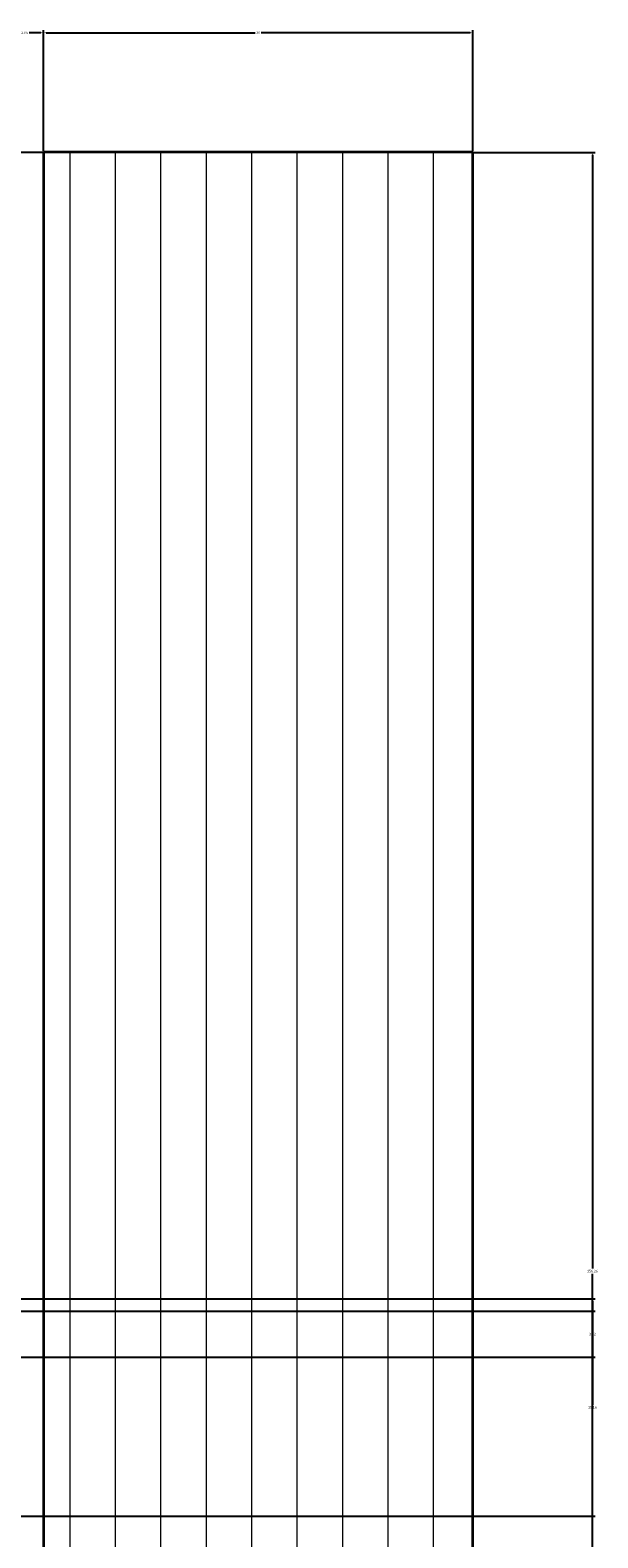
# Model space of a CAD drawing. Units: millimetres. Extents: x 446512 to 447461, y 70395 to 70610.
# Tile 21 of 39: x 446748 to 446788, y 70473 to 70578. Entities that reach past the tile are written whole.
import ezdxf

# ---------------------------------------------------------------- set-up
doc = ezdxf.new("R2010")
doc.units = ezdxf.units.MM
for name, color, linetype, lineweight in [('A-ANNO-DIMS', 2, 'Continuous', 18), ('A-FURN', 7, 'Continuous', 35), ('A-FURN-PATT', 38, 'Continuous', 13)]:
    doc.layers.add(name, color=color, linetype=linetype, lineweight=lineweight)
doc.styles.get("Standard").update_dxf_attribs({"font": 'arial.ttf'})
doc.dimstyles.get("Standard").update_dxf_attribs({"dimtxt": 0.18, "dimasz": 0.18, "dimexe": 0.18, "dimexo": 0.0625, "dimgap": 0.09, "dimtad": 0, "dimtih": 1, "dimtoh": 1, "dimdec": 4, "dimzin": 0, "dimdsep": 46, "dimtxsty": 'Standard', "dimcen": 0.09, "dimadec": 0, "dimazin": 0, "dimtfac": 1, "dimtdec": 4, "dimtofl": 0, "dimtmove": 0, "dimatfit": 3, "dimfxl": 1, "dimtolj": 1, "dimtzin": 0, "dimarcsym": 0})

# ---------------------------------------------------------------- blocks, each defined once
blk = doc.blocks.new('*D15')
at = {"layer": 'A-ANNO-DIMS', "color": 0, "lineweight": -2, "transparency": 16777216}
for p, q in [((446746.57, 70533.44), (446746.57, 70578.17)), ((446749.22, 70569.71), (446749.22, 70578.17)), ((446746.75, 70577.99), (446747.57, 70577.99)), ((446749.04, 70577.99), (446748.22, 70577.99))]:
    blk.add_line(p, q, dxfattribs=at)
at = {"layer": 'A-ANNO-DIMS', "color": 0, "transparency": 16777216}
for points in [[(446746.75, 70578.02), (446746.75, 70577.96), (446746.57, 70577.99)], [(446749.04, 70578.02), (446749.04, 70577.96), (446749.22, 70577.99)]]:
    blk.add_solid(points, dxfattribs=at)
at = {"layer": 'Defpoints', "color": 0, "transparency": 16777216}
for p in [(446749.22, 70577.99), (446749.22, 70569.64), (446746.57, 70533.38)]:
    blk.add_point(p, dxfattribs=at)
at = {"layer": 'A-ANNO-DIMS', "color": 0, "transparency": 16777216, "insert": (446747.9, 70577.99), "char_height": 0.18, "attachment_point": 5}
blk.add_mtext('\\A1;2.65', dxfattribs=at)
blk = doc.blocks.new('*D16')
at = {"layer": 'A-ANNO-DIMS', "color": 0, "lineweight": -2, "transparency": 16777216}
for p, q in [((446749.22, 70569.71), (446749.22, 70578.17)), ((446779.22, 70569.71), (446779.22, 70578.17)), ((446749.4, 70577.99), (446764, 70577.99)), ((446779.04, 70577.99), (446764.44, 70577.99))]:
    blk.add_line(p, q, dxfattribs=at)
at = {"layer": 'A-ANNO-DIMS', "color": 0, "transparency": 16777216}
for points in [[(446749.4, 70578.02), (446749.4, 70577.96), (446749.22, 70577.99)], [(446779.04, 70578.02), (446779.04, 70577.96), (446779.22, 70577.99)]]:
    blk.add_solid(points, dxfattribs=at)
at = {"layer": 'Defpoints', "color": 0, "transparency": 16777216}
for p in [(446779.22, 70577.99), (446749.22, 70569.64), (446779.22, 70569.64)]:
    blk.add_point(p, dxfattribs=at)
at = {"layer": 'A-ANNO-DIMS', "color": 0, "transparency": 16777216, "insert": (446764.22, 70577.99), "char_height": 0.18, "attachment_point": 5}
blk.add_mtext('\\A1;30', dxfattribs=at)
blk = doc.blocks.new('*D17')
at = {"layer": 'A-ANNO-DIMS', "color": 0, "lineweight": -2, "transparency": 16777216}
for p, q in [((446779.29, 70569.64), (446787.75, 70569.64)), ((446787.57, 70569.46), (446787.57, 70491.7)), ((446787.57, 70413.56), (446787.57, 70491.33)), ((446779.29, 70413.38), (446787.75, 70413.38))]:
    blk.add_line(p, q, dxfattribs=at)
at = {"layer": 'A-ANNO-DIMS', "color": 0, "transparency": 16777216}
for points in [[(446787.54, 70569.46), (446787.6, 70569.46), (446787.57, 70569.64)], [(446787.54, 70413.56), (446787.6, 70413.56), (446787.57, 70413.38)]]:
    blk.add_solid(points, dxfattribs=at)
at = {"layer": 'Defpoints', "color": 0, "transparency": 16777216}
for p in [(446779.22, 70569.64), (446787.57, 70569.64), (446779.22, 70413.38)]:
    blk.add_point(p, dxfattribs=at)
at = {"layer": 'A-ANNO-DIMS', "color": 0, "transparency": 16777216, "insert": (446787.57, 70491.51), "char_height": 0.18, "attachment_point": 5}
blk.add_mtext('\\A1;156.26', dxfattribs=at)
blk = doc.blocks.new('*D24')
at = {"layer": 'A-ANNO-DIMS', "color": 0, "lineweight": -2, "transparency": 16777216}
for p, q in [((446749.16, 70569.64), (446678.04, 70569.64)), ((446678.22, 70569.46), (446678.22, 70551.7)), ((446678.22, 70533.56), (446678.22, 70551.33)), ((446686.51, 70533.38), (446678.04, 70533.38))]:
    blk.add_line(p, q, dxfattribs=at)
at = {"layer": 'A-ANNO-DIMS', "color": 0, "transparency": 16777216}
for points in [[(446678.19, 70569.46), (446678.25, 70569.46), (446678.22, 70569.64)], [(446678.19, 70533.56), (446678.25, 70533.56), (446678.22, 70533.38)]]:
    blk.add_solid(points, dxfattribs=at)
at = {"layer": 'Defpoints', "color": 0, "transparency": 16777216}
for p in [(446678.22, 70569.64), (446749.22, 70569.64), (446686.57, 70533.38)]:
    blk.add_point(p, dxfattribs=at)
at = {"layer": 'A-ANNO-DIMS', "color": 0, "transparency": 16777216, "insert": (446678.22, 70551.51), "char_height": 0.18, "attachment_point": 5}
blk.add_mtext('\\A1;36.26', dxfattribs=at)
blk = doc.blocks.new('*D30')
at = {"layer": 'A-ANNO-DIMS', "color": 0, "lineweight": -2, "transparency": 16777216}
for p, q in [((446743.64, 70489.58), (446787.75, 70489.58)), ((446787.57, 70489.4), (446787.57, 70482.18)), ((446787.57, 70474.58), (446787.57, 70481.81)), ((446743.64, 70474.4), (446787.75, 70474.4))]:
    blk.add_line(p, q, dxfattribs=at)
at = {"layer": 'A-ANNO-DIMS', "color": 0, "transparency": 16777216}
for points in [[(446787.54, 70489.4), (446787.6, 70489.4), (446787.57, 70489.58)], [(446787.54, 70474.58), (446787.6, 70474.58), (446787.57, 70474.4)]]:
    blk.add_solid(points, dxfattribs=at)
at = {"layer": 'Defpoints', "color": 0, "transparency": 16777216}
for p in [(446743.58, 70489.58), (446787.57, 70489.58), (446743.58, 70474.4)]:
    blk.add_point(p, dxfattribs=at)
at = {"layer": 'A-ANNO-DIMS', "color": 0, "transparency": 16777216, "insert": (446787.57, 70481.99), "char_height": 0.18, "attachment_point": 5}
blk.add_mtext('\\A1;15.18', dxfattribs=at)
blk = doc.blocks.new('*D35')
at = {"layer": 'A-ANNO-DIMS', "color": 0, "lineweight": -2, "transparency": 16777216}
for p, q in [((446742.78, 70488.72), (446787.75, 70488.72)), ((446787.57, 70488.54), (446787.57, 70487.3)), ((446787.57, 70485.68), (446787.57, 70486.93)), ((446739.38, 70485.5), (446787.75, 70485.5))]:
    blk.add_line(p, q, dxfattribs=at)
at = {"layer": 'A-ANNO-DIMS', "color": 0, "transparency": 16777216}
for points in [[(446787.54, 70488.54), (446787.6, 70488.54), (446787.57, 70488.72)], [(446787.54, 70485.68), (446787.6, 70485.68), (446787.57, 70485.5)]]:
    blk.add_solid(points, dxfattribs=at)
at = {"layer": 'Defpoints', "color": 0, "transparency": 16777216}
for p in [(446742.72, 70488.72), (446739.32, 70485.5), (446787.57, 70485.5)]:
    blk.add_point(p, dxfattribs=at)
at = {"layer": 'A-ANNO-DIMS', "color": 0, "transparency": 16777216, "insert": (446787.57, 70487.11), "char_height": 0.18, "attachment_point": 5}
blk.add_mtext('\\A1;3.22', dxfattribs=at)

msp = doc.modelspace()

# ---------------------------------------------------------------- hatches: boundary and pattern name
at = {"layer": 'A-FURN-PATT'}
h = msp.add_hatch(dxfattribs=at)
h.set_pattern_fill('ANSI31', color=256, angle=45)
h.paths.add_polyline_path([(446779.2235, 70569.6449), (446749.2235, 70569.6449), (446749.2235, 70413.3815), (446779.2235, 70413.3815)])

# ---------------------------------------------------------------- linework, layer by layer
at = {"layer": 'A-FURN'}
for p, q in [((446779.2235, 70569.6449), (446749.2235, 70569.6449)), ((446749.2235, 70569.6449), (446749.2235, 70413.3815)), ((446779.2235, 70413.3815), (446779.2235, 70569.6449))]:
    msp.add_line(p, q, dxfattribs=at)

# ---------------------------------------------------------------- dimensions: what is measured, and where the dimension line sits
at = {"layer": 'A-ANNO-DIMS'}
for base, p1, p2, override, picture, middle in [((446749.2235, 70577.9949), (446746.5728, 70533.3816), (446749.2235, 70569.6449), {"dimdec": 2, "dimlfac": 1, "dimrnd": 0, "dimzin": 0, "dimdsep": 46, "dimlunit": 2}, '*D15', (446747.8982, 70577.9949)), ((446779.2235, 70577.9949), (446749.2235, 70569.6449), (446779.2235, 70569.6449), {"dimdec": 0, "dimlfac": 1, "dimrnd": 0, "dimzin": 0, "dimdsep": 46, "dimlunit": 2}, '*D16', (446764.2235, 70577.9949))]:
    dim = msp.add_linear_dim(base=base, p1=p1, p2=p2, dimstyle='Standard', override=override, dxfattribs=at)
    dim.commit()
    dim.dimension.update_dxf_attribs({"geometry": picture, "text_midpoint": middle})
for base, p1, p2, picture, middle in [((446678.2228, 70569.6449), (446686.5728, 70533.3816), (446749.2235, 70569.6449), '*D24', (446678.2228, 70551.5132)), ((446787.5735, 70569.6449), (446779.2235, 70413.3815), (446779.2235, 70569.6449), '*D17', (446787.5735, 70491.5132)), ((446787.5735, 70485.5045), (446742.7192, 70488.7221), (446739.3181, 70485.5045), '*D35', (446787.5735, 70487.1133)), ((446787.5735, 70489.5845), (446743.5815, 70474.4047), (446743.5815, 70489.5845), '*D30', (446787.5735, 70481.9946))]:
    dim = msp.add_linear_dim(base=base, p1=p1, p2=p2, angle=90, dimstyle='Standard', override={"dimdec": 2, "dimlfac": 1, "dimrnd": 0, "dimzin": 0, "dimdsep": 46, "dimlunit": 2}, dxfattribs=at)
    dim.commit()
    dim.dimension.update_dxf_attribs({"geometry": picture, "text_midpoint": middle})

doc.saveas('drawing.dxf')
